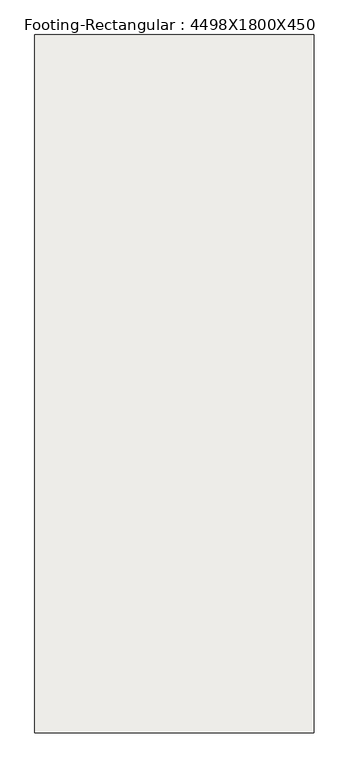
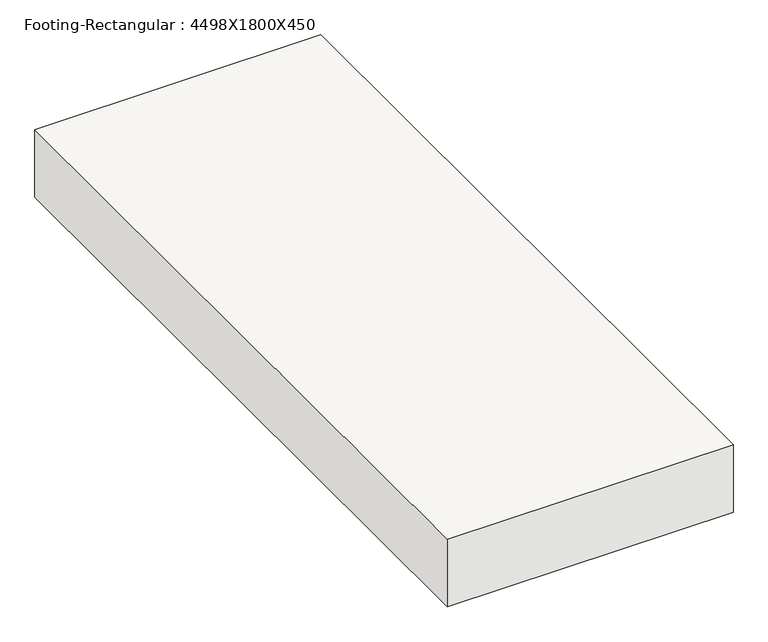
"""IFC4 building model written with IfcOpenShell, lengths in millimetres: slab geometry, Footing-Rectangular : 4498X1800X450."""

from ifc_helpers import new_model, si_unit, frame, origin, place, context, project, spatial, polyline, outline, extrude, source, transform, mapped, element, save


def footing_rectangular_4498x1800x450_c2833046(model_context):
    return source(origin(), model_context, "Body", "SweptSolid", [
        extrude(outline(polyline([(900.0, 2249.0), (900.0, -2249.0), (-900.0, -2249.0), (-900.0, 2249.0), (900.0, 2249.0)])), frame((0.0, 0.0, -450.0), z_axis=(0.0, 0.0, 1.0), x_axis=(1.0, 0.0, 0.0)), (0.0, 0.0, 1.0), 450.0),
    ])


if __name__ == "__main__":
    model = new_model("IFC4")
    model_context = context("Model", 3, world=origin())
    ifc_project = project(units=[si_unit("LENGTHUNIT", "METRE", prefix="MILLI")], contexts=[model_context])
    site = spatial("IfcSite", under=ifc_project)
    building = spatial("IfcBuilding", under=site)
    placement = place(None, origin())
    footing_rectangular_4498x1800x450_shape = footing_rectangular_4498x1800x450_c2833046(model_context)
    element("IfcSlab", 1, ObjectType="Footing-Rectangular : 4498X1800X450", at=placement, inside=building, context=model_context, shape_type="MappedRepresentation", body=[
        mapped(footing_rectangular_4498x1800x450_shape, transform((0.0, 0.0, 0.0), x_axis=(1.0, 0.0, 0.0), y_axis=(0.0, 1.0, 0.0), z_axis=(0.0, 0.0, 1.0))),
    ])
    save(model, "model.ifc")

# Revit data of these elements
# Type "Footing-Rectangular : 4498X1800X450"
#   Width = 5' - 10.86614"
#   Length = 14' - 9.08661"
#   Foundation Thickness = 1' - 5.71654"
#   Structural Material [instance default] = Concrete - Cast-in-Place Concrete
#   Assembly Code = ""
# Element 1 (IfcSlab, "Footing-Rectangular : 4498X1800X450")
#   Materials on its faces: "Concrete - Cast-in-Place Concrete"
# Materials
#   "Concrete - Cast-in-Place Concrete": class "Concrete", colour RGB 192 192 192, transparency 0, Cost = 0
